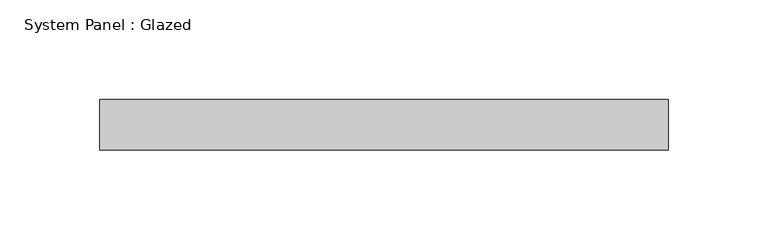
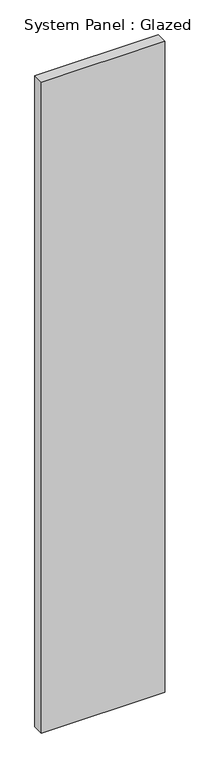
"""IFC4 building model written with IfcOpenShell, lengths in millimetres: plate geometry, System Panel : Glazed."""

from ifc_helpers import new_model, si_unit, origin, origin_with_axes, place, context, project, spatial, polyline, outline, extrude, source, transform, mapped, element, save


def system_panel_glazed_6f8e0303(model_context):
    return source(origin(), model_context, "Body", "SweptSolid", [
        extrude(outline(polyline([(142.875, 19.05), (-142.875, 19.05), (-142.875, 44.45), (142.875, 44.45), (142.875, 19.05)])), origin_with_axes(), (0.0, 0.0, 1.0), 1592.9882445),
    ])


if __name__ == "__main__":
    model = new_model("IFC4")
    model_context = context("Model", 3, world=origin())
    ifc_project = project(units=[si_unit("LENGTHUNIT", "METRE", prefix="MILLI")], contexts=[model_context])
    site = spatial("IfcSite", under=ifc_project)
    building = spatial("IfcBuilding", under=site)
    placement = place(None, origin())
    system_panel_glazed_shape = system_panel_glazed_6f8e0303(model_context)
    element("IfcPlate", 1, ObjectType="System Panel : Glazed", at=placement, inside=building, context=model_context, shape_type="MappedRepresentation", body=[
        mapped(system_panel_glazed_shape, transform((0.0, 0.0, 0.0), x_axis=(1.0, 0.0, 0.0), y_axis=(0.0, 1.0, 0.0), z_axis=(0.0, 0.0, 1.0))),
    ])
    save(model, "model.ifc")

# Revit data of these elements
# Type "System Panel : Glazed"
#   Construction Type Id = "GSP4R"
#   Analytic Construction = "1/8 in Pilkington single glazing"
#   Visual Light Transmittance = 0.9
#   Solar Heat Gain Coefficient = 0.86
#   Heat Transfer Coefficient (U) = 1.18115 BTU/(h·ft²·°F)
#   Define Thermal Properties by = 1
# Element 1 (IfcPlate, "System Panel : Glazed")
#   Materials on its faces: "Glass"
# Materials
#   "Glass": class "Glass", colour RGB 0 128 192, transparency 0.75, Description = "Soda Lime Glass", Cost = 0
